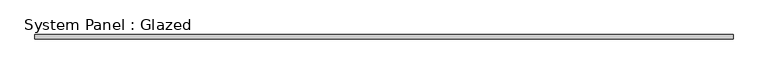
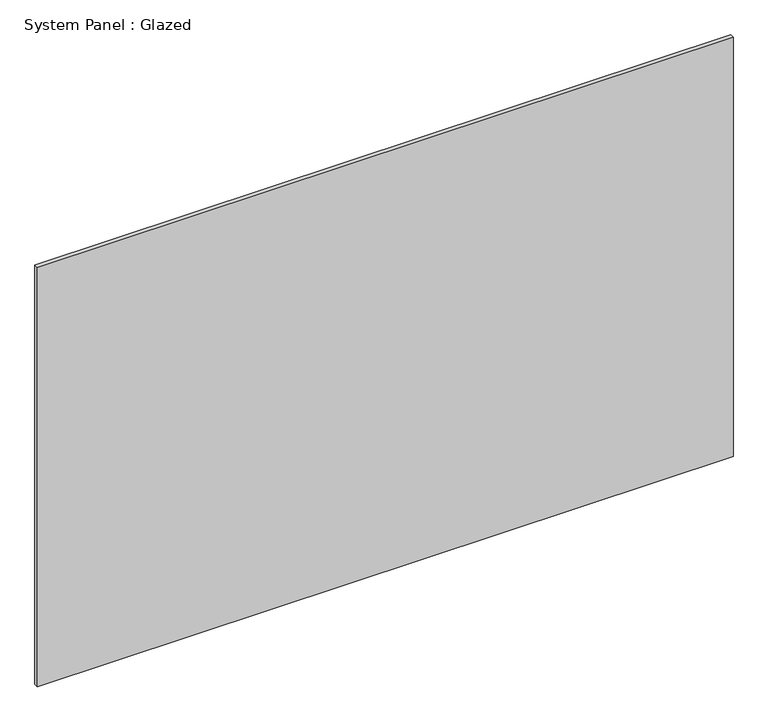
"""IFC4 building model written with IfcOpenShell, lengths in millimetres: plate geometry, System Panel : Glazed."""

from ifc_helpers import new_model, si_unit, origin, origin_with_axes, place, context, project, spatial, polyline, outline, extrude, source, transform, mapped, element, save


def system_panel_glazed_54db570c(model_context):
    return source(origin(), model_context, "Body", "SweptSolid", [
        extrude(outline(polyline([(2052.0644396, 19.05), (-2052.0644396, 19.05), (-2052.0644396, 44.45), (2052.0644396, 44.45), (2052.0644396, 19.05)])), origin_with_axes(), (0.0, 0.0, 1.0), 2616.2),
    ])


if __name__ == "__main__":
    model = new_model("IFC4")
    model_context = context("Model", 3, world=origin())
    ifc_project = project(units=[si_unit("LENGTHUNIT", "METRE", prefix="MILLI")], contexts=[model_context])
    site = spatial("IfcSite", under=ifc_project)
    building = spatial("IfcBuilding", under=site)
    placement = place(None, origin())
    system_panel_glazed_shape = system_panel_glazed_54db570c(model_context)
    element("IfcPlate", 1, ObjectType="System Panel : Glazed", at=placement, inside=building, context=model_context, shape_type="MappedRepresentation", body=[
        mapped(system_panel_glazed_shape, transform((0.0, 0.0, 0.0), x_axis=(1.0, 0.0, 0.0), y_axis=(0.0, 1.0, 0.0), z_axis=(0.0, 0.0, 1.0))),
    ])
    save(model, "model.ifc")

# Revit data of these elements
# Type "System Panel : Glazed"
#   Construction Type Id = "GSP4R"
#   Analytic Construction = "1/8 in Pilkington single glazing"
#   Visual Light Transmittance = 0.9
#   Solar Heat Gain Coefficient = 0.86
#   Heat Transfer Coefficient (U) = 1.18115 BTU/(h·ft²·°F)
# Element 1 (IfcPlate, "System Panel : Glazed")
#   Materials on its faces: "Glass"
# Materials
#   "Glass": class "Glass", colour RGB 0 128 192, transparency 0.75, Description = "Soda Lime Glass", Cost = 0
